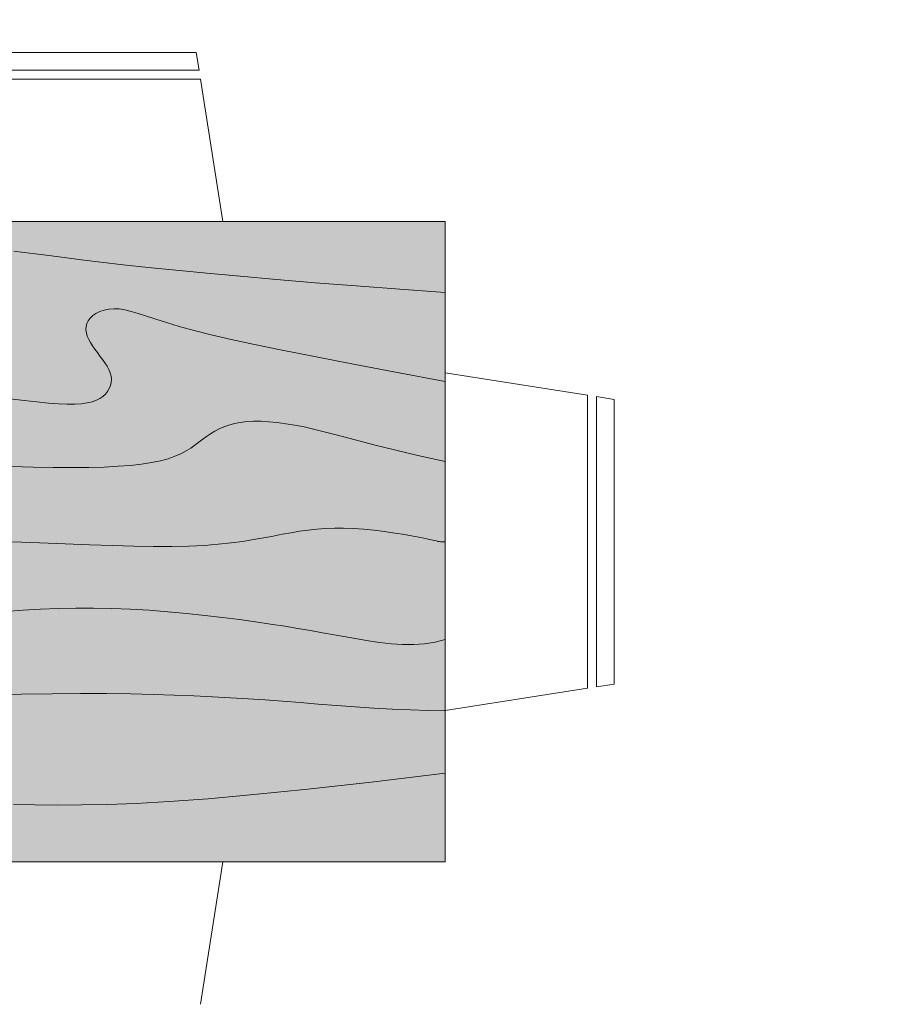
# Model space of a CAD drawing. Units: inches. Extents: x 2419 to 2878, y 1068 to 1713.
# Tile 6 of 20: x 2541 to 2574, y 1312 to 1349. Entities that reach past the tile are written whole.
import ezdxf

# ---------------------------------------------------------------- set-up
doc = ezdxf.new("R2010")
doc.units = ezdxf.units.IN
for name, color, linetype, lineweight in [('A-ANNO-DIMS', 2, 'Continuous', 18), ('A-FLOR-PRKG-PATT', 1, 'Continuous', 13), ('A-FURN', 8, 'Continuous', 18), ('A-FURN-PATT', 254, 'Continuous', 13)]:
    doc.layers.add(name, color=color, linetype=linetype, lineweight=lineweight)
doc.layers.add('A-WALL-PATT', color=18, linetype='Continuous', lineweight=13, true_color=0x000000)
doc.styles.get("Standard").update_dxf_attribs({"font": 'arial.ttf'})
doc.dimstyles.new('ISO-25', dxfattribs={"dimtxt": 12.5, "dimasz": 2.5, "dimexe": 1.25, "dimexo": 0.625, "dimtad": 1, "dimdec": 0, "dimlunit": 4, "dimtxsty": 'Standard', "dimblk": 'ARCHTICK', "dimcen": 2.5, "dimse1": 1, "dimse2": 1, "dimclrd": 4, "dimadec": 0, "dimazin": 0, "dimtfac": 1, "dimtdec": 0, "dimtmove": 0, "dimatfit": 3, "dimfxl": 1, "dimarcsym": 0})

# ---------------------------------------------------------------- blocks, each defined once
blk = doc.blocks.new('Dining Set - 36 x 72 in.')
for p, q in [((6, 27.5), (22, 27.5)), ((22.1563, 26.49966), (22, 27.5)), ((22.1584, 26.5), (5.8466, 26.5)), ((5.7696, 26), (22.2392, 26)), ((23.4848, 17.99762), (22.2345, 25.99926)), ((36, 18), (-36, 18)), ((36, -18), (36, 18)), ((44.0006, 8.23428), (35.9976, 9.48474)), ((44, 8.23041), (44, -8.23915)), ((44.5, -8.15843), (44.5, 8.15338)), ((45.5, 8), (44.5005, 8.15617)), ((45.5, 8), (45.5, -8)), ((35.9976, -9.48476), (43.9993, -8.2345)), ((44.4997, -8.15631), (45.5, -8)), ((-36, -18), (36, -18)), ((23.4848, -17.99762), (22.2345, -25.99928))]:
    blk.add_line(p, q)
for points in [[(11.75, 16.33333), (12.3184, 16.26318), (12.9694, 16.17838), (13.7151, 16.07991), (14.5677, 15.96875), (15.5395, 15.84586), (16.6426, 15.71224), (17.8893, 15.56884), (19.2917, 15.41666), (20.859, 15.25667), (22.5879, 15.08984), (24.4721, 14.91715), (26.5052, 14.73958), (28.6809, 14.5581), (30.9929, 14.3737), (33.4347, 14.18733), (36, 14)], [(11.5312, 8.03125), (12.3267, 7.93603), (13.043, 7.85547), (13.6831, 7.79248), (14.25, 7.75), (14.7471, 7.7303), (15.1797, 7.73307), (15.5537, 7.75732), (15.875, 7.80208), (16.1494, 7.86637), (16.3828, 7.94922), (16.5811, 8.04964), (16.75, 8.16666), (16.8944, 8.29915), (17.0143, 8.44531), (17.1089, 8.60319), (17.1771, 8.77083), (17.218, 8.94629), (17.2305, 9.1276), (17.2137, 9.31282), (17.1667, 9.5), (17.0895, 9.6875), (16.987, 9.875), (16.8649, 10.0625), (16.7292, 10.25), (16.5856, 10.4375), (16.4401, 10.625), (16.2985, 10.8125), (16.1667, 11), (16.05, 11.18733), (15.9518, 11.3737), (15.8752, 11.5581), (15.8229, 11.73958), (15.798, 11.91715), (15.8034, 12.08984), (15.842, 12.25667), (15.9167, 12.41666), (16.0295, 12.56836), (16.1784, 12.70833), (16.3605, 12.83268), (16.5729, 12.9375), (16.8127, 13.01888), (17.0768, 13.07291), (17.3625, 13.0957), (17.6667, 13.08333), (17.9894, 13.03312), (18.3418, 12.94726), (18.7382, 12.82918), (19.1927, 12.68229), (19.7195, 12.51001), (20.3327, 12.31575), (21.0465, 12.10294), (21.875, 11.875), (22.8357, 11.63354), (23.959, 11.37304), (25.2786, 11.08618), (26.8282, 10.76562), (28.6414, 10.40405), (30.752, 9.99414), (33.1936, 9.52856), (36, 9)], [(11.6309, 4.22819), (12.8281, 4.19531), (13.9551, 4.17415), (15, 4.16666), (15.954, 4.17448), (16.819, 4.19791), (17.6001, 4.23698), (18.3021, 4.29166), (18.9299, 4.36198), (19.4883, 4.44791), (19.9823, 4.54948), (20.4167, 4.66666), (20.7969, 4.79899), (21.1302, 4.94401), (21.4245, 5.09879), (21.6875, 5.26041), (21.9271, 5.42594), (22.1511, 5.59245), (22.3672, 5.757), (22.5834, 5.91666), (22.8065, 6.06868), (23.0404, 6.21093), (23.2879, 6.34147), (23.5521, 6.45833), (23.8358, 6.55957), (24.142, 6.64323), (24.4735, 6.70735), (24.8334, 6.75), (25.2235, 6.76969), (25.642, 6.76692), (26.0858, 6.74267), (26.5521, 6.69791), (27.0379, 6.63362), (27.5404, 6.55078), (28.0565, 6.45036), (28.5834, 6.33333), (29.1242, 6.19987), (29.7071, 6.04687), (30.3661, 5.87044), (31.1354, 5.66666), (32.0493, 5.43164), (33.142, 5.16146), (34.4475, 4.85221), (36, 4.5)], [(11.6667, 0), (13.1899, -0.06201), (14.6341, -0.1211), (15.9982, -0.17432), (17.2813, -0.21875), (18.4823, -0.25147), (19.6003, -0.26953), (20.6343, -0.27002), (21.5834, -0.25), (22.4481, -0.20768), (23.2357, -0.14584), (23.9549, -0.06836), (24.6146, 0.02083), (25.2235, 0.11784), (25.7904, 0.21875), (26.3241, 0.31966), (26.8334, 0.41666), (27.3265, 0.50618), (27.8099, 0.58593), (28.2894, 0.65397), (28.7709, 0.70833), (29.2601, 0.74707), (29.763, 0.76823), (30.2855, 0.76985), (30.8334, 0.75), (31.4088, 0.70784), (31.9994, 0.64713), (32.589, 0.57275), (33.1615, 0.48958), (33.7008, 0.4025), (34.1908, 0.3164), (34.6153, 0.23616), (34.9584, 0.16666), (35.2099, 0.11165), (35.3848, 0.07031), (35.504, 0.04069), (35.5886, 0.02083), (35.6594, 0.00879), (35.7377, 0.0026), (35.8442, 0.00032), (36, 0)], [(11.2734, -3.91407), (12.2647, -3.84603), (13.25, -3.79167), (14.2354, -3.75293), (15.2266, -3.73177), (16.2295, -3.73015), (17.25, -3.75), (18.2912, -3.79248), (19.3451, -3.85547), (20.4009, -3.93604), (21.4479, -4.03125), (22.4754, -4.13819), (23.4727, -4.25391), (24.4289, -4.37549), (25.3334, -4.5), (26.1785, -4.62492), (26.9694, -4.74935), (27.7145, -4.87281), (28.4219, -4.99479), (29.1, -5.11483), (29.7572, -5.23242), (30.4016, -5.34709), (31.0417, -5.45834), (31.6837, -5.56437), (32.3262, -5.65821), (32.9658, -5.73153), (33.599, -5.77604), (34.2224, -5.78345), (34.8327, -5.74545), (35.4264, -5.65373), (36, -5.5)], [(10.3021, -8.60677), (12.1712, -8.56543), (13.8958, -8.54167), (15.4876, -8.53353), (16.9583, -8.53907), (18.3197, -8.55632), (19.5834, -8.58334), (20.7616, -8.61841), (21.8685, -8.66081), (22.9188, -8.71004), (23.9271, -8.76563), (24.9081, -8.82707), (25.8763, -8.89388), (26.8465, -8.96558), (27.8334, -9.04167), (28.8474, -9.12118), (29.8828, -9.20117), (30.93, -9.27824), (31.9792, -9.34896), (33.0205, -9.40991), (34.0443, -9.45768), (35.0407, -9.48885), (36, -9.5)], [(11.7192, -14.76164), (12.929, -14.78711), (14.1965, -14.79794), (15.5417, -14.79167), (16.9933, -14.76424), (18.6152, -14.70508), (20.4804, -14.60197), (22.6615, -14.44271), (25.2312, -14.21509), (28.2624, -13.9069), (31.8277, -13.50594), (36, -13)]]:
    blk.add_lwpolyline(points)
blk = doc.blocks.new('_ArchTick')
at = {"color": 0, "linetype": 'ByBlock', "const_width": 0.15}
blk.add_lwpolyline([(-0.5, -0.5), (0.5, 0.5)], dxfattribs=at)
blk = doc.blocks.new('*D26')
at = {"layer": 'A-ANNO-DIMS', "color": 4, "lineweight": -2, "transparency": 16777216}
for p, q in [((2502.769, 1356.79), (2563.458, 1356.79)), ((2563.458, 1356.79), (2733.724, 1356.79))]:
    blk.add_line(p, q, dxfattribs=at)
at = {"layer": 'Defpoints', "color": 0, "transparency": 16777216}
for p in [(2563.458, 1356.79), (2502.769, 1347.687), (2563.458, 1347.687)]:
    blk.add_point(p, dxfattribs=at)
at = {"layer": 'A-ANNO-DIMS', "color": 4, "lineweight": -2, "transparency": 16777216, "xscale": 2.5, "yscale": 2.5, "zscale": 2.5, "rotation": 180}
blk.add_blockref('_ArchTick', (2502.769, 1356.79), dxfattribs=at)
at = {"layer": 'A-ANNO-DIMS', "color": 4, "lineweight": -2, "transparency": 16777216, "xscale": 2.5, "yscale": 2.5, "zscale": 2.5}
blk.add_blockref('_ArchTick', (2563.458, 1356.79), dxfattribs=at)
at = {"layer": 'A-ANNO-DIMS', "color": 0, "transparency": 16777216, "insert": (2649.841, 1363.878), "char_height": 12.5, "attachment_point": 5}
blk.add_mtext('DINING SET 5\'-0 1/2"', dxfattribs=at)
blk = doc.blocks.new('*D43')
at = {"layer": 'A-ANNO-DIMS', "color": 4, "lineweight": -2, "transparency": 16777216}
blk.add_line((2480.514, 1079.925), (2557.299, 1079.925), dxfattribs=at)
at = {"layer": 'Defpoints', "color": 0, "transparency": 16777216}
for p in [(2480.514, 1408.813), (2557.299, 1408.813), (2557.299, 1079.925)]:
    blk.add_point(p, dxfattribs=at)
at = {"layer": 'A-ANNO-DIMS', "color": 4, "lineweight": -2, "transparency": 16777216, "xscale": 2.5, "yscale": 2.5, "zscale": 2.5, "rotation": 180}
blk.add_blockref('_ArchTick', (2480.514, 1079.925), dxfattribs=at)
at = {"layer": 'A-ANNO-DIMS', "color": 4, "lineweight": -2, "transparency": 16777216, "xscale": 2.5, "yscale": 2.5, "zscale": 2.5}
blk.add_blockref('_ArchTick', (2557.299, 1079.925), dxfattribs=at)
at = {"layer": 'A-ANNO-DIMS', "color": 0, "transparency": 16777216, "insert": (2518.907, 1086.932), "char_height": 12.5, "attachment_point": 5}
blk.add_mtext('6\'-5"', dxfattribs=at)
blk = doc.blocks.new('*D44')
at = {"layer": 'A-ANNO-DIMS', "color": 4, "lineweight": -2, "transparency": 16777216}
for p, q in [((2557.299, 1079.925), (2585.818, 1079.925)), ((2585.818, 1079.925), (2652.136, 1079.925))]:
    blk.add_line(p, q, dxfattribs=at)
at = {"layer": 'Defpoints', "color": 0, "transparency": 16777216}
for p in [(2557.299, 1408.813), (2585.818, 1408.813), (2585.818, 1079.925)]:
    blk.add_point(p, dxfattribs=at)
at = {"layer": 'A-ANNO-DIMS', "color": 4, "lineweight": -2, "transparency": 16777216, "xscale": 2.5, "yscale": 2.5, "zscale": 2.5, "rotation": 180}
blk.add_blockref('_ArchTick', (2557.299, 1079.925), dxfattribs=at)
at = {"layer": 'A-ANNO-DIMS', "color": 4, "lineweight": -2, "transparency": 16777216, "xscale": 2.5, "yscale": 2.5, "zscale": 2.5}
blk.add_blockref('_ArchTick', (2585.818, 1079.925), dxfattribs=at)
at = {"layer": 'A-ANNO-DIMS', "color": 0, "transparency": 16777216, "insert": (2620.227, 1087.013), "char_height": 12.5, "attachment_point": 5}
blk.add_mtext('2\'-4 1/2"', dxfattribs=at)
blk = doc.blocks.new('*D47')
at = {"layer": 'A-ANNO-DIMS', "color": 4, "lineweight": -2, "transparency": 16777216}
for p, q in [((2444.314, 1376.561), (2444.314, 1357.976)), ((2444.314, 1357.976), (2444.314, 1293.048))]:
    blk.add_line(p, q, dxfattribs=at)
at = {"layer": 'Defpoints', "color": 0, "transparency": 16777216}
for p in [(2632.514, 1376.561), (2444.314, 1357.976), (2632.514, 1357.976)]:
    blk.add_point(p, dxfattribs=at)
at = {"layer": 'A-ANNO-DIMS', "color": 4, "lineweight": -2, "transparency": 16777216, "xscale": 2.5, "yscale": 2.5, "zscale": 2.5}
for p, rotation in [((2444.314, 1376.561), 90), ((2444.314, 1357.976), 270)]:
    blk.add_blockref('_ArchTick', p, dxfattribs=dict(at, rotation=rotation))
at = {"layer": 'A-ANNO-DIMS', "color": 0, "transparency": 16777216, "insert": (2437.226, 1324.262), "char_height": 12.5, "attachment_point": 5, "rotation": 90}
blk.add_mtext('1\'-6 1/2"', dxfattribs=at)
blk = doc.blocks.new('*D56')
at = {"layer": 'A-ANNO-DIMS', "color": 4, "lineweight": -2, "transparency": 16777216}
for p, q in [((2480.514, 1079.925), (2503.967, 1079.925)), ((2503.967, 1079.925), (2578.607, 1079.925))]:
    blk.add_line(p, q, dxfattribs=at)
at = {"layer": 'Defpoints', "color": 0, "transparency": 16777216}
for p in [(2480.514, 1507.813), (2503.967, 1494.852), (2503.967, 1079.925)]:
    blk.add_point(p, dxfattribs=at)
at = {"layer": 'A-ANNO-DIMS', "color": 4, "lineweight": -2, "transparency": 16777216, "xscale": 2.5, "yscale": 2.5, "zscale": 2.5, "rotation": 180}
blk.add_blockref('_ArchTick', (2480.514, 1079.925), dxfattribs=at)
at = {"layer": 'A-ANNO-DIMS', "color": 4, "lineweight": -2, "transparency": 16777216, "xscale": 2.5, "yscale": 2.5, "zscale": 2.5}
blk.add_blockref('_ArchTick', (2503.967, 1079.925), dxfattribs=at)
at = {"layer": 'A-ANNO-DIMS', "color": 0, "transparency": 16777216, "insert": (2542.537, 1087.013), "char_height": 12.5, "attachment_point": 5}
blk.add_mtext('1\'-11 1/2"', dxfattribs=at)
blk = doc.blocks.new('*D59')
at = {"layer": 'A-ANNO-DIMS', "color": 4, "lineweight": -2, "transparency": 16777216}
blk.add_line((2480.514, 1079.925), (2589.514, 1079.925), dxfattribs=at)
at = {"layer": 'Defpoints', "color": 0, "transparency": 16777216}
for p in [(2480.514, 1414.813), (2589.514, 1414.813), (2589.514, 1079.925)]:
    blk.add_point(p, dxfattribs=at)
at = {"layer": 'A-ANNO-DIMS', "color": 4, "lineweight": -2, "transparency": 16777216, "xscale": 2.5, "yscale": 2.5, "zscale": 2.5, "rotation": 180}
blk.add_blockref('_ArchTick', (2480.514, 1079.925), dxfattribs=at)
at = {"layer": 'A-ANNO-DIMS', "color": 4, "lineweight": -2, "transparency": 16777216, "xscale": 2.5, "yscale": 2.5, "zscale": 2.5}
blk.add_blockref('_ArchTick', (2589.514, 1079.925), dxfattribs=at)
at = {"layer": 'A-ANNO-DIMS', "color": 0, "transparency": 16777216, "insert": (2535.014, 1086.932), "char_height": 12.5, "attachment_point": 5}
blk.add_mtext('9\'-1"', dxfattribs=at)

msp = doc.modelspace()

# ---------------------------------------------------------------- hatches: boundary and pattern name
at = {"layer": 'A-FLOR-PRKG-PATT'}
h = msp.add_hatch(color=256, dxfattribs=at)
h.dxf.hatch_style = 1
edge = h.paths.add_edge_path()
edge.add_ellipse((2561.374, 1279.453), major_axis=(3.988, 0), ratio=0.842304, start_angle=0.6466, end_angle=90)
edge.add_line((2561.374, 1282.813), (2511.571, 1282.813))
edge.add_ellipse((2511.571, 1279.453), major_axis=(3.988, 0), ratio=0.842304, start_angle=90, end_angle=179.3534)
edge.add_ellipse((10560.892, 1188.617), major_axis=(-8054.031, 0), ratio=0.84230387, start_angle=-0.6465541, end_angle=-0.6282372)
edge.add_ellipse((2509.23, 1276.906), major_axis=(1.687, 0), ratio=0.842304, start_angle=179.3718, end_angle=248.4648)
edge.add_ellipse((10560.329, 1188.617), major_axis=(8052.293, 0), ratio=0.84230387, start_angle=179.3534459, end_angle=179.3813568, ccw=False)
edge.add_ellipse((2511.008, 1279.453), major_axis=(2.25, 0), ratio=0.842304, start_angle=90, end_angle=179.3534, ccw=False)
edge.add_line((2511.008, 1281.348), (2561.936, 1281.348))
edge.add_ellipse((2561.936, 1279.453), major_axis=(-2.25, 0), ratio=0.842304, start_angle=180.6466, end_angle=270, ccw=False)
edge.add_ellipse((-5487.385, 1188.617), major_axis=(8052.293, 0), ratio=0.84230387, start_angle=0.5282715, end_angle=0.6465541, ccw=False)
edge.add_ellipse((2563.715, 1276.906), major_axis=(-1.687, 0), ratio=0.842304, start_angle=111.5352, end_angle=180.6282)
edge.add_ellipse((-5487.947, 1188.617), major_axis=(-8054.031, 0), ratio=0.84230387, start_angle=180.6282372, end_angle=180.6465541)
edge = h.paths.add_edge_path()
edge.add_ellipse((2564.908, 1261.91), major_axis=(-1.125, 0), ratio=0.842304, start_angle=180, end_angle=270)
edge.add_line((2564.908, 1262.857), (2564.426, 1262.857))
edge.add_ellipse((-5487.385, 1188.617), major_axis=(8052.293, 0), ratio=0.84230387, start_angle=0.3838668, end_angle=0.5282715, ccw=False)
edge.add_line((2564.654, 1242.564), (2564.908, 1242.564))
edge.add_ellipse((2564.908, 1243.512), major_axis=(-1.125, 0), ratio=0.842304, start_angle=90, end_angle=180)
edge.add_line((2566.033, 1243.512), (2566.033, 1261.91))
edge = h.paths.add_edge_path()
edge.add_ellipse((2564.908, 1174.989), major_axis=(1.125, 0), ratio=0.842304, start_angle=0, end_angle=90)
edge.add_line((2564.908, 1175.936), (2564.894, 1175.936))
edge.add_ellipse((-5487.385, 1188.617), major_axis=(8052.293, 0), ratio=0.84230387, start_angle=-0.1349866, end_angle=-0.0902291, ccw=False)
edge.add_ellipse((2163.343, 1170.913), major_axis=(401.537, 0), ratio=0.8423039, start_angle=-2.17995, end_angle=-0.13561, ccw=False)
edge.add_line((2564.47, 1155.643), (2564.908, 1155.643))
edge.add_ellipse((2564.908, 1156.591), major_axis=(-1.125, 0), ratio=0.842304, start_angle=90, end_angle=180)
edge.add_line((2566.033, 1156.591), (2566.033, 1174.989))
h.paths.add_polyline_path([(2574.476, 1207.448), (2633.94, 1207.448), (2633.94, 1217.366), (2574.476, 1217.366)], flags=9)
h.paths.add_polyline_path([(2574.454, 1217.828), (2610.472, 1217.828), (2610.472, 1227.879), (2574.454, 1227.879)], flags=9)
h.paths.add_polyline_path([(2672.426, 1304.02), (2718.617, 1304.02), (2718.617, 1313.939), (2672.426, 1313.939)], flags=9)
h.paths.add_polyline_path([(2672.404, 1314.4), (2750.128, 1314.4), (2750.128, 1324.451), (2672.404, 1324.451)], flags=9)
h.paths.add_polyline_path([(2500.432, 1374.444), (2544.803, 1374.444), (2544.803, 1384.362), (2500.432, 1384.362)], flags=9)
h.paths.add_polyline_path([(2500.41, 1384.824), (2566.075, 1384.824), (2566.075, 1394.875), (2500.41, 1394.875)], flags=9)
h.paths.add_polyline_path([(2738.933, 1376.749), (2778.273, 1376.749), (2778.273, 1386.667), (2738.933, 1386.667)], flags=9)
h.paths.add_polyline_path([(2659.12, 1357.8), (2703.492, 1357.8), (2703.492, 1367.718), (2659.12, 1367.718)], flags=9)
h.paths.add_polyline_path([(2659.098, 1368.18), (2694.114, 1368.18), (2694.114, 1378.23), (2659.098, 1378.23)], flags=9)
h.paths.add_polyline_path([(2730.123, 1466.067), (2769.463, 1466.067), (2769.463, 1475.986), (2730.123, 1475.986)], flags=9)
h.paths.add_polyline_path([(2730.101, 1476.447), (2765.117, 1476.447), (2765.117, 1486.498), (2730.101, 1486.498)], flags=9)
h.paths.add_polyline_path([(2730.382, 1518.647), (2761.48, 1518.647), (2761.48, 1528.566), (2730.382, 1528.566)], flags=9)
h.paths.add_polyline_path([(2730.361, 1529.028), (2780.958, 1529.028), (2780.958, 1539.072), (2730.361, 1539.072)], flags=9)
h.paths.add_polyline_path([(2629.32, 1455.189), (2688.784, 1455.189), (2688.784, 1465.107), (2629.32, 1465.107)], flags=9)
h.paths.add_polyline_path([(2629.298, 1465.569), (2681.902, 1465.569), (2681.902, 1475.62), (2629.298, 1475.62)], flags=9)
h.paths.add_polyline_path([(2513.229, 1456.484), (2562.631, 1456.484), (2562.631, 1466.402), (2513.229, 1466.402)], flags=9)
h.paths.add_polyline_path([(2513.208, 1466.865), (2556.26, 1466.865), (2556.26, 1476.909), (2513.208, 1476.909)], flags=9)
h.paths.add_polyline_path([(2488.87, 1521.538), (2519.968, 1521.538), (2519.968, 1531.456), (2488.87, 1531.456)], flags=9)
h.paths.add_polyline_path([(2536.549, 1543.507), (2580.923, 1543.507), (2580.923, 1553.432), (2536.549, 1553.432)], flags=9)
h.paths.add_polyline_path([(2536.557, 1553.921), (2573.525, 1553.921), (2573.525, 1563.8), (2536.557, 1563.8)], flags=9)
at = {"layer": 'A-FURN-PATT'}
h = msp.add_hatch(color=256, dxfattribs=at)
h.dxf.hatch_style = 1
h.paths.add_polyline_path([(2541.329, 1340.193), (2541.763, 1340.136), (2542.26, 1340.071), (2542.829, 1339.996), (2543.477, 1339.914), (2544.213, 1339.825), (2545.044, 1339.73), (2545.979, 1339.628), (2547.025, 1339.521), (2548.178, 1339.41), (2549.434, 1339.295), (2550.79, 1339.177), (2552.241, 1339.056), (2553.783, 1338.933), (2555.412, 1338.808), (2557.123, 1338.683), (2557.123, 1341.351), (2509.104, 1341.351), (2509.104, 1339.35), (2512.321, 1339.335), (2515.235, 1339.293), (2517.872, 1339.227), (2520.258, 1339.142), (2522.419, 1339.041), (2524.38, 1338.928), (2526.167, 1338.808), (2527.806, 1338.683), (2529.318, 1338.559), (2530.71, 1338.437), (2531.983, 1338.32), (2533.138, 1338.211), (2534.177, 1338.112), (2535.102, 1338.027), (2535.914, 1337.957), (2536.615, 1337.905), (2537.208, 1337.874), (2537.702, 1337.862), (2538.108, 1337.868), (2538.435, 1337.891), (2538.695, 1337.93), (2538.897, 1337.983), (2539.052, 1338.05), (2539.171, 1338.128), (2539.263, 1338.216), (2539.33, 1338.313), (2539.376, 1338.416), (2539.401, 1338.524), (2539.407, 1338.634), (2539.398, 1338.745), (2539.374, 1338.855), (2539.338, 1338.961), (2539.292, 1339.063), (2539.238, 1339.16), (2539.211, 1339.204), (2538.872, 1339.739), (2539.045, 1340.125), (2539.381, 1340.287), (2539.76, 1340.325), (2540.185, 1340.315), (2540.752, 1340.264)])
h.paths.add_polyline_path([(2557.123, 1329.334), (2556.881, 1329.353), (2556.861, 1329.358), (2556.848, 1329.36), (2556.516, 1329.438), (2556.428, 1329.458), (2556.199, 1329.504), (2555.916, 1329.558), (2555.589, 1329.615), (2555.23, 1329.673), (2554.848, 1329.728), (2554.455, 1329.778), (2554.061, 1329.819), (2553.677, 1329.847), (2553.311, 1329.86), (2552.963, 1329.859), (2552.628, 1329.845), (2552.301, 1329.819), (2551.98, 1329.783), (2551.66, 1329.737), (2551.338, 1329.684), (2551.009, 1329.624), (2550.353, 1329.499), (2549.707, 1329.384), (2549.089, 1329.301), (2548.61, 1329.249), (2548.085, 1329.208), (2547.508, 1329.18), (2546.875, 1329.166), (2546.185, 1329.167), (2545.44, 1329.179), (2544.639, 1329.201), (2543.783, 1329.23), (2542.873, 1329.266), (2541.91, 1329.305), (2540.894, 1329.346), (2539.824, 1329.388), (2538.691, 1329.428), (2537.484, 1329.464), (2536.191, 1329.496), (2534.802, 1329.521), (2533.305, 1329.538), (2531.69, 1329.545), (2529.946, 1329.541), (2528.058, 1329.523), (2526.009, 1329.488), (2523.776, 1329.432), (2521.338, 1329.35), (2518.673, 1329.238), (2515.761, 1329.092), (2512.578, 1328.907), (2509.104, 1328.68), (2509.104, 1325.012), (2514.984, 1325.136), (2519.719, 1325.261), (2523.464, 1325.384), (2526.371, 1325.505), (2528.595, 1325.623), (2530.288, 1325.738), (2531.604, 1325.85), (2532.697, 1325.956), (2533.694, 1326.058), (2534.628, 1326.154), (2535.506, 1326.245), (2536.333, 1326.331), (2537.118, 1326.412), (2537.867, 1326.488), (2538.586, 1326.558), (2539.282, 1326.623), (2539.963, 1326.683), (2540.632, 1326.736), (2541.293, 1326.782), (2541.95, 1326.818), (2542.607, 1326.844), (2543.268, 1326.858), (2543.937, 1326.859), (2544.618, 1326.846), (2545.312, 1326.817), (2546.015, 1326.775), (2546.719, 1326.721), (2547.418, 1326.658), (2548.103, 1326.587), (2548.768, 1326.509), (2549.406, 1326.428), (2550.009, 1326.345), (2550.572, 1326.262), (2551.1, 1326.179), (2551.597, 1326.097), (2552.069, 1326.015), (2552.521, 1325.935), (2552.959, 1325.857), (2553.389, 1325.78), (2553.816, 1325.706), (2554.244, 1325.636), (2554.672, 1325.573), (2555.099, 1325.524), (2555.521, 1325.494), (2555.937, 1325.489), (2556.344, 1325.515), (2556.74, 1325.576), (2557.123, 1325.678)])
h.paths.add_polyline_path([(2557.123, 1335.349), (2555.251, 1335.701), (2553.623, 1336.012), (2552.215, 1336.285), (2551.006, 1336.526), (2549.972, 1336.74), (2549.092, 1336.931), (2548.343, 1337.105), (2547.702, 1337.266), (2547.15, 1337.418), (2546.674, 1337.56), (2546.265, 1337.69), (2545.913, 1337.805), (2545.61, 1337.903), (2545.346, 1337.981), (2545.111, 1338.039), (2544.896, 1338.072), (2544.693, 1338.08), (2544.502, 1338.065), (2544.326, 1338.029), (2544.166, 1337.975), (2544.025, 1337.905), (2543.903, 1337.822), (2543.804, 1337.729), (2543.729, 1337.627), (2543.679, 1337.521), (2543.653, 1337.409), (2543.649, 1337.294), (2543.666, 1337.176), (2543.701, 1337.055), (2543.752, 1336.932), (2543.818, 1336.808), (2543.895, 1336.683), (2543.983, 1336.558), (2544.078, 1336.433), (2544.175, 1336.307), (2544.271, 1336.182), (2544.361, 1336.057), (2544.442, 1335.932), (2544.511, 1335.807), (2544.562, 1335.682), (2544.594, 1335.557), (2544.605, 1335.434), (2544.597, 1335.313), (2544.569, 1335.196), (2544.524, 1335.084), (2544.461, 1334.979), (2544.381, 1334.881), (2544.284, 1334.793), (2544.172, 1334.715), (2544.039, 1334.648), (2543.884, 1334.593), (2543.701, 1334.55), (2543.487, 1334.52), (2543.237, 1334.504), (2542.949, 1334.502), (2542.617, 1334.515), (2542.239, 1334.543), (2541.812, 1334.585), (2541.334, 1334.639), (2540.804, 1334.703), (2540.219, 1334.774), (2539.577, 1334.851), (2538.876, 1334.932), (2538.115, 1335.015), (2537.292, 1335.099), (2536.409, 1335.183), (2535.465, 1335.268), (2534.465, 1335.356), (2533.408, 1335.446), (2532.297, 1335.539), (2531.133, 1335.636), (2529.918, 1335.738), (2528.635, 1335.843), (2527.193, 1335.945), (2525.484, 1336.036), (2523.398, 1336.106), (2520.826, 1336.148), (2517.659, 1336.152), (2513.788, 1336.111), (2509.104, 1336.016), (2509.104, 1333.015), (2512.629, 1332.904), (2515.728, 1332.821), (2518.445, 1332.76), (2520.824, 1332.716), (2522.909, 1332.685), (2524.743, 1332.663), (2526.37, 1332.645), (2527.834, 1332.626), (2529.173, 1332.602), (2530.407, 1332.574), (2531.551, 1332.542), (2532.62, 1332.507), (2533.63, 1332.47), (2534.594, 1332.43), (2535.529, 1332.389), (2536.448, 1332.348), (2537.364, 1332.306), (2538.272, 1332.266), (2539.164, 1332.228), (2540.033, 1332.195), (2540.87, 1332.166), (2541.669, 1332.144), (2542.42, 1332.13), (2543.117, 1332.125), (2543.754, 1332.131), (2544.33, 1332.146), (2544.851, 1332.172), (2545.32, 1332.209), (2545.738, 1332.256), (2546.111, 1332.313), (2546.44, 1332.381), (2546.73, 1332.459), (2546.983, 1332.547), (2547.206, 1332.644), (2547.402, 1332.747), (2547.577, 1332.855), (2547.737, 1332.965), (2547.886, 1333.076), (2548.031, 1333.186), (2548.175, 1333.292), (2548.324, 1333.394), (2548.48, 1333.489), (2548.645, 1333.576), (2548.821, 1333.654), (2549.01, 1333.721), (2549.214, 1333.777), (2549.435, 1333.82), (2549.675, 1333.848), (2549.936, 1333.861), (2550.215, 1333.859), (2550.511, 1333.843), (2550.822, 1333.813), (2551.146, 1333.771), (2551.481, 1333.715), (2551.825, 1333.648), (2552.176, 1333.57), (2552.537, 1333.481), (2552.926, 1333.379), (2553.365, 1333.262), (2553.878, 1333.126), (2554.488, 1332.969), (2555.217, 1332.789), (2556.087, 1332.583), (2557.123, 1332.348)])
h.paths.add_polyline_path([(2543.679, 1337.521), (2543.729, 1337.627), (2543.804, 1337.729), (2543.903, 1337.822), (2544.025, 1337.905), (2544.166, 1337.975), (2544.326, 1338.029), (2544.502, 1338.065), (2544.693, 1338.08), (2544.896, 1338.072), (2545.111, 1338.039), (2545.346, 1337.981), (2545.61, 1337.903), (2545.913, 1337.805), (2546.265, 1337.69), (2546.674, 1337.56), (2547.15, 1337.418), (2547.702, 1337.266), (2548.343, 1337.105), (2549.092, 1336.931), (2549.972, 1336.74), (2551.006, 1336.526), (2552.215, 1336.285), (2553.623, 1336.012), (2555.251, 1335.701), (2557.123, 1335.349), (2557.123, 1338.683), (2555.412, 1338.808), (2553.783, 1338.933), (2552.241, 1339.056), (2550.79, 1339.177), (2549.434, 1339.295), (2548.178, 1339.41), (2547.025, 1339.521), (2545.979, 1339.628), (2545.044, 1339.73), (2544.213, 1339.825), (2543.477, 1339.914), (2542.829, 1339.996), (2542.26, 1340.071), (2541.763, 1340.136), (2541.329, 1340.193), (2540.95, 1340.24), (2540.618, 1340.276), (2540.33, 1340.302), (2540.08, 1340.318), (2539.866, 1340.323), (2539.683, 1340.318), (2539.527, 1340.302), (2539.395, 1340.276), (2539.282, 1340.24), (2539.186, 1340.193), (2539.105, 1340.137), (2539.04, 1340.073), (2538.991, 1340.003), (2538.957, 1339.928), (2538.939, 1339.849), (2538.936, 1339.767), (2538.949, 1339.684), (2538.977, 1339.6), (2539.018, 1339.516), (2539.067, 1339.431), (2539.123, 1339.343), (2539.222, 1339.189), (2539.323, 1339.007), (2539.374, 1338.855), (2539.398, 1338.745), (2539.407, 1338.634), (2539.401, 1338.524), (2539.376, 1338.416), (2539.33, 1338.313), (2539.263, 1338.216), (2539.171, 1338.128), (2539.052, 1338.05), (2538.897, 1337.983), (2538.695, 1337.93), (2538.435, 1337.891), (2538.108, 1337.868), (2537.702, 1337.862), (2537.208, 1337.874), (2536.615, 1337.905), (2535.914, 1337.957), (2535.102, 1338.027), (2534.177, 1338.112), (2533.138, 1338.211), (2531.983, 1338.32), (2530.71, 1338.437), (2529.318, 1338.559), (2527.806, 1338.683), (2526.167, 1338.808), (2524.38, 1338.928), (2522.419, 1339.041), (2520.258, 1339.142), (2517.872, 1339.227), (2515.235, 1339.293), (2512.321, 1339.335), (2509.104, 1339.35), (2509.104, 1336.016), (2513.788, 1336.111), (2517.659, 1336.152), (2520.826, 1336.148), (2523.398, 1336.106), (2525.484, 1336.036), (2527.193, 1335.945), (2528.635, 1335.843), (2529.918, 1335.738), (2531.133, 1335.636), (2532.297, 1335.539), (2533.408, 1335.446), (2534.465, 1335.356), (2535.465, 1335.268), (2536.409, 1335.183), (2537.292, 1335.099), (2538.115, 1335.015), (2538.876, 1334.932), (2539.577, 1334.851), (2540.219, 1334.774), (2540.804, 1334.703), (2541.334, 1334.639), (2541.812, 1334.585), (2542.239, 1334.543), (2542.617, 1334.515), (2542.949, 1334.502), (2543.237, 1334.504), (2543.487, 1334.52), (2543.701, 1334.55), (2543.884, 1334.593), (2544.039, 1334.648), (2544.172, 1334.715), (2544.284, 1334.793), (2544.381, 1334.881), (2544.461, 1334.979), (2544.524, 1335.084), (2544.569, 1335.196), (2544.597, 1335.313), (2544.605, 1335.434), (2544.594, 1335.557), (2544.562, 1335.682), (2544.511, 1335.807), (2544.442, 1335.932), (2544.361, 1336.057), (2544.271, 1336.182), (2544.175, 1336.307), (2544.078, 1336.433), (2543.983, 1336.558), (2543.895, 1336.683), (2543.818, 1336.808), (2543.752, 1336.932), (2543.701, 1337.055), (2543.666, 1337.176), (2543.649, 1337.294), (2543.653, 1337.409)])
h.paths.add_polyline_path([(2557.123, 1332.348), (2556.087, 1332.583), (2555.217, 1332.789), (2554.488, 1332.969), (2553.878, 1333.126), (2553.365, 1333.262), (2552.926, 1333.379), (2552.537, 1333.481), (2552.176, 1333.57), (2551.825, 1333.648), (2551.481, 1333.715), (2551.146, 1333.771), (2550.822, 1333.813), (2550.511, 1333.843), (2550.215, 1333.859), (2549.936, 1333.861), (2549.675, 1333.848), (2549.435, 1333.82), (2549.214, 1333.777), (2549.01, 1333.721), (2548.821, 1333.654), (2548.645, 1333.576), (2548.48, 1333.489), (2548.324, 1333.394), (2548.175, 1333.292), (2548.031, 1333.186), (2547.886, 1333.076), (2547.737, 1332.965), (2547.577, 1332.855), (2547.402, 1332.747), (2547.206, 1332.644), (2546.983, 1332.547), (2546.73, 1332.459), (2546.44, 1332.381), (2546.111, 1332.313), (2545.738, 1332.256), (2545.32, 1332.209), (2544.851, 1332.172), (2544.33, 1332.146), (2543.754, 1332.131), (2543.117, 1332.125), (2542.42, 1332.13), (2541.669, 1332.144), (2540.87, 1332.166), (2540.033, 1332.195), (2539.164, 1332.228), (2538.272, 1332.266), (2537.364, 1332.306), (2536.448, 1332.348), (2535.529, 1332.389), (2534.594, 1332.43), (2533.63, 1332.47), (2532.62, 1332.507), (2531.551, 1332.542), (2530.407, 1332.574), (2529.173, 1332.602), (2527.834, 1332.626), (2526.37, 1332.645), (2524.743, 1332.663), (2522.909, 1332.685), (2520.824, 1332.716), (2518.445, 1332.76), (2515.728, 1332.821), (2512.629, 1332.904), (2509.104, 1333.015), (2509.104, 1328.68), (2512.578, 1328.907), (2515.761, 1329.092), (2518.673, 1329.238), (2521.338, 1329.35), (2523.776, 1329.432), (2526.009, 1329.488), (2528.058, 1329.523), (2529.946, 1329.541), (2531.69, 1329.545), (2533.305, 1329.538), (2534.802, 1329.521), (2536.191, 1329.496), (2537.484, 1329.464), (2538.691, 1329.428), (2539.824, 1329.388), (2540.894, 1329.346), (2541.91, 1329.305), (2542.873, 1329.266), (2543.783, 1329.23), (2544.639, 1329.201), (2545.44, 1329.179), (2546.185, 1329.167), (2546.875, 1329.166), (2547.508, 1329.18), (2548.085, 1329.208), (2548.61, 1329.249), (2549.089, 1329.301), (2549.529, 1329.36), (2549.936, 1329.425), (2550.314, 1329.492), (2550.67, 1329.56), (2551.009, 1329.624), (2551.338, 1329.684), (2551.66, 1329.737), (2551.98, 1329.783), (2552.301, 1329.819), (2552.628, 1329.845), (2552.963, 1329.859), (2553.311, 1329.86), (2553.677, 1329.847), (2554.061, 1329.819), (2554.455, 1329.778), (2554.848, 1329.728), (2555.23, 1329.673), (2555.589, 1329.615), (2555.916, 1329.558), (2556.199, 1329.504), (2556.428, 1329.458), (2556.596, 1329.421), (2556.712, 1329.393), (2556.792, 1329.374), (2556.848, 1329.36), (2556.895, 1329.352), (2556.948, 1329.348), (2557.019, 1329.347), (2557.123, 1329.346)])
h.paths.add_polyline_path([(2557.123, 1323.011), (2556.483, 1323.018), (2555.818, 1323.039), (2555.136, 1323.071), (2554.441, 1323.111), (2553.741, 1323.159), (2553.043, 1323.21), (2552.352, 1323.263), (2551.676, 1323.316), (2551.018, 1323.367), (2550.371, 1323.415), (2549.725, 1323.46), (2549.071, 1323.501), (2548.398, 1323.538), (2547.698, 1323.57), (2546.96, 1323.599), (2546.174, 1323.622), (2545.331, 1323.64), (2544.423, 1323.652), (2543.442, 1323.655), (2542.381, 1323.65), (2541.231, 1323.634), (2539.984, 1323.606), (2538.633, 1323.566), (2537.171, 1323.511), (2535.566, 1323.441), (2533.7, 1323.357), (2531.431, 1323.262), (2528.619, 1323.157), (2525.121, 1323.044), (2520.797, 1322.925), (2515.505, 1322.802), (2509.104, 1322.677), (2509.104, 1319.676), (2513.047, 1319.786), (2516.418, 1319.868), (2519.287, 1319.925), (2521.724, 1319.961), (2523.797, 1319.978), (2525.575, 1319.981), (2527.13, 1319.972), (2528.528, 1319.954), (2529.831, 1319.931), (2531.052, 1319.903), (2532.199, 1319.871), (2533.277, 1319.836), (2534.29, 1319.798), (2535.246, 1319.759), (2536.148, 1319.718), (2537.004, 1319.676), (2537.819, 1319.635), (2538.606, 1319.595), (2539.377, 1319.558), (2540.147, 1319.527), (2540.929, 1319.502), (2541.736, 1319.485), (2542.581, 1319.477), (2543.479, 1319.482), (2544.447, 1319.5), (2545.528, 1319.539), (2546.772, 1319.608), (2548.227, 1319.714), (2549.941, 1319.866), (2551.962, 1320.072), (2554.34, 1320.339), (2557.123, 1320.677)], flags=17)
h.paths.add_polyline_path([(2557.123, 1325.678), (2556.74, 1325.576), (2556.344, 1325.515), (2555.937, 1325.489), (2555.521, 1325.494), (2555.099, 1325.524), (2554.672, 1325.573), (2554.244, 1325.636), (2553.816, 1325.706), (2553.389, 1325.78), (2552.959, 1325.857), (2552.521, 1325.935), (2552.069, 1326.015), (2551.597, 1326.097), (2551.1, 1326.179), (2550.572, 1326.262), (2550.009, 1326.345), (2549.406, 1326.428), (2548.768, 1326.509), (2548.103, 1326.587), (2547.418, 1326.658), (2546.719, 1326.721), (2546.015, 1326.775), (2545.312, 1326.817), (2544.618, 1326.846), (2543.937, 1326.859), (2543.268, 1326.858), (2542.607, 1326.844), (2541.95, 1326.818), (2541.293, 1326.782), (2540.632, 1326.736), (2539.963, 1326.683), (2539.282, 1326.623), (2538.586, 1326.558), (2537.867, 1326.488), (2537.118, 1326.412), (2536.333, 1326.331), (2535.506, 1326.245), (2534.628, 1326.154), (2533.694, 1326.058), (2532.697, 1325.956), (2531.604, 1325.85), (2530.288, 1325.738), (2528.595, 1325.623), (2526.371, 1325.505), (2523.464, 1325.384), (2519.719, 1325.261), (2514.984, 1325.136), (2509.104, 1325.012), (2509.104, 1319.676), (2513.047, 1319.786), (2516.418, 1319.868), (2519.287, 1319.925), (2521.724, 1319.961), (2523.797, 1319.978), (2525.575, 1319.981), (2527.13, 1319.972), (2528.528, 1319.954), (2529.831, 1319.931), (2531.052, 1319.903), (2532.199, 1319.871), (2533.277, 1319.836), (2534.29, 1319.798), (2535.246, 1319.759), (2536.148, 1319.718), (2537.004, 1319.676), (2537.819, 1319.635), (2538.606, 1319.595), (2539.377, 1319.558), (2540.147, 1319.527), (2540.929, 1319.502), (2541.736, 1319.485), (2542.581, 1319.477), (2543.479, 1319.482), (2544.447, 1319.5), (2545.528, 1319.539), (2546.772, 1319.608), (2548.227, 1319.714), (2549.941, 1319.866), (2551.962, 1320.072), (2554.34, 1320.339), (2557.123, 1320.677)])
h.paths.add_polyline_path([(2557.123, 1320.677), (2554.34, 1320.339), (2551.962, 1320.072), (2549.941, 1319.866), (2548.227, 1319.714), (2546.772, 1319.608), (2545.528, 1319.539), (2544.447, 1319.5), (2543.479, 1319.482), (2542.581, 1319.477), (2541.736, 1319.485), (2540.929, 1319.502), (2540.147, 1319.527), (2539.377, 1319.558), (2538.606, 1319.595), (2537.819, 1319.635), (2537.004, 1319.676), (2536.148, 1319.718), (2535.246, 1319.759), (2534.29, 1319.798), (2533.277, 1319.836), (2532.199, 1319.871), (2531.052, 1319.903), (2529.831, 1319.931), (2528.528, 1319.954), (2527.13, 1319.972), (2525.575, 1319.981), (2523.797, 1319.978), (2521.724, 1319.961), (2519.287, 1319.925), (2516.418, 1319.868), (2513.047, 1319.786), (2509.104, 1319.676), (2509.104, 1317.342), (2557.123, 1317.342)])
h = msp.add_hatch(color=256, dxfattribs=at)
h.dxf.hatch_style = 1
h.paths.add_polyline_path([(2557.123, 1323.011), (2556.483, 1323.018), (2555.818, 1323.039), (2555.136, 1323.071), (2554.441, 1323.111), (2553.741, 1323.159), (2553.043, 1323.21), (2552.352, 1323.263), (2551.676, 1323.316), (2551.018, 1323.367), (2550.371, 1323.415), (2549.725, 1323.46), (2549.071, 1323.501), (2548.398, 1323.538), (2547.698, 1323.57), (2546.96, 1323.599), (2546.174, 1323.622), (2545.331, 1323.64), (2544.423, 1323.652), (2543.442, 1323.655), (2542.381, 1323.65), (2541.231, 1323.634), (2539.984, 1323.606), (2538.633, 1323.566), (2537.171, 1323.511), (2535.566, 1323.441), (2533.7, 1323.357), (2531.431, 1323.262), (2528.619, 1323.157), (2525.121, 1323.044), (2520.797, 1322.925), (2515.505, 1322.802), (2509.104, 1322.677), (2509.104, 1319.676), (2513.047, 1319.786), (2516.418, 1319.868), (2519.287, 1319.925), (2521.724, 1319.961), (2523.797, 1319.978), (2525.575, 1319.981), (2527.13, 1319.972), (2528.528, 1319.954), (2529.831, 1319.931), (2531.052, 1319.903), (2532.199, 1319.871), (2533.277, 1319.836), (2534.29, 1319.798), (2535.246, 1319.759), (2536.148, 1319.718), (2537.004, 1319.676), (2537.819, 1319.635), (2538.606, 1319.595), (2539.377, 1319.558), (2540.147, 1319.527), (2540.929, 1319.502), (2541.736, 1319.485), (2542.581, 1319.477), (2543.479, 1319.482), (2544.447, 1319.5), (2545.528, 1319.539), (2546.772, 1319.608), (2548.227, 1319.714), (2549.941, 1319.866), (2551.962, 1320.072), (2554.34, 1320.339), (2557.123, 1320.677)])
at = {"layer": 'A-WALL-PATT'}
h = msp.add_hatch(color=256, dxfattribs=at)
h.dxf.hatch_style = 1
h.paths.add_polyline_path([(2780.514, 1577.813), (2471.514, 1577.813), (2471.514, 1121.813), (2780.514, 1121.813)])
h.paths.add_polyline_path([(2480.514, 1568.813), (2771.514, 1568.813), (2771.514, 1130.813), (2480.514, 1130.813)], flags=16)
h.paths.add_polyline_path([(2528.514, 1568.813), (2528.514, 1512.813), (2594.514, 1512.813), (2594.514, 1414.813), (2596.568, 1414.813), (2596.568, 1441.609), (2597.816, 1441.609), (2597.816, 1441.582, -0.384016), (2625.035, 1414.813), (2725.514, 1414.813), (2725.514, 1567.545), (2728.302, 1567.545), (2746.887, 1567.545), (2746.887, 1566.732), (2746.87, 1566.732, -0.367216), (2730.514, 1549.092), (2730.514, 1512.813), (2750.853, 1512.813), (2750.853, 1510.025, -0.401453), (2733.081, 1491.458), (2733.081, 1491.44), (2732.268, 1491.44), (2732.268, 1507.813), (2730.514, 1507.813), (2730.514, 1408.813), (2736.514, 1408.813), (2736.514, 1349.813), (2632.514, 1349.813), (2632.514, 1408.813), (2528.514, 1408.813), (2528.514, 1414.813), (2503.967, 1414.813), (2503.967, 1494.852), (2558.379, 1494.852), (2558.379, 1507.813), (2529.965, 1507.813, -0.414214), (2530.821, 1506.957), (2530.821, 1497.257, -0.414214), (2529.965, 1496.401), (2514.559, 1496.401, -0.414214), (2513.703, 1497.257), (2513.703, 1506.957, -0.414214), (2514.559, 1507.813), (2528.514, 1507.813), (2528.514, 1512.813), (2480.514, 1512.813)], flags=0)
h.paths.add_polyline_path([(2516.262, 1507.813), (2528.262, 1507.813), (2528.262, 1505.813), (2523.417, 1505.813), (2524.074, 1504.675), (2529.394, 1504.675, -0.414214), (2529.965, 1504.104), (2529.965, 1497.828, -0.414214), (2529.394, 1497.257), (2515.13, 1497.257, -0.414214), (2514.559, 1497.828), (2514.559, 1504.104, -0.414214), (2515.13, 1504.675), (2520.689, 1504.675), (2521.342, 1505.813), (2516.262, 1505.813)], flags=0)
h.paths.add_polyline_path([(2522.016, 1505.531), (2522.817, 1507.318, -0.65506), (2522.254, 1506.063), (2522.195, 1505.93), (2522.425, 1505.531)], flags=0)
h.paths.add_polyline_path([(2522.833, 1500.966, -1), (2521.691, 1500.966, -1)], flags=0)
h.paths.add_polyline_path([(2522.547, 1500.966, -1), (2521.977, 1500.966, -1)], flags=0)
h.paths.add_polyline_path([(2482.005, 1470.633), (2499.894, 1470.633), (2499.894, 1448.272), (2482.005, 1448.272), (2482.005, 1452.744), (2481.26, 1452.744), (2481.26, 1449.763), (2480.514, 1449.763), (2480.514, 1469.142), (2481.26, 1469.142), (2481.26, 1466.16), (2482.005, 1466.16)], flags=0)
h.paths.add_polyline_path([(2488.713, 1466.16, -1), (2484.241, 1466.16, -1)], flags=0)
h.paths.add_polyline_path([(2496.167, 1466.16, -1), (2490.204, 1466.16, -1)], flags=0)
h.paths.add_polyline_path([(2487.968, 1466.16, -1), (2484.987, 1466.16, -1)], flags=0)
h.paths.add_polyline_path([(2495.422, 1466.16, -1), (2490.949, 1466.16, -1)], flags=0)
h.paths.add_polyline_path([(2487.223, 1466.16, -1), (2485.732, 1466.16, -1)], flags=0)
h.paths.add_polyline_path([(2494.676, 1466.16, -1), (2491.695, 1466.16, -1)], flags=0)
h.paths.add_polyline_path([(2499.108, 1468.005, -1), (2497.977, 1468.005, -1)], flags=0)
h.paths.add_polyline_path([(2493.931, 1466.16, -1), (2492.44, 1466.16, -1)], flags=0)
h.paths.add_polyline_path([(2499.372, 1463.71, -1), (2498.166, 1463.71, -1)], flags=0)
h.paths.add_polyline_path([(2484.241, 1461.688), (2496.167, 1461.688), (2496.167, 1457.216), (2484.241, 1457.216)], flags=0)
h.paths.add_polyline_path([(2484.987, 1460.943), (2495.422, 1460.943), (2495.422, 1457.961), (2484.987, 1457.961)], flags=0)
h.paths.add_polyline_path([(2586.88, 1510.025), (2587.693, 1510.025), (2587.693, 1491.44), (2586.88, 1491.44)], flags=0)
h.paths.add_polyline_path([(2499.259, 1459.415, -1), (2498.203, 1459.415, -1)], flags=0)
h.paths.add_polyline_path([(2489.459, 1452.744, -1), (2483.496, 1452.744, -1)], flags=0)
h.paths.add_polyline_path([(2557.299, 1408.813), (2557.299, 1413.091, -0.401453), (2584.57, 1441.582), (2584.57, 1441.609), (2585.818, 1441.609), (2585.818, 1413.091), (2585.818, 1408.813)], flags=0)
h.paths.add_polyline_path([(2488.713, 1452.744, -1), (2484.241, 1452.744, -1)], flags=0)
h.paths.add_polyline_path([(2495.422, 1452.744, -1), (2490.949, 1452.744, -1)], flags=0)
h.paths.add_polyline_path([(2487.968, 1452.744, -1), (2484.987, 1452.744, -1)], flags=0)
h.paths.add_polyline_path([(2494.676, 1452.744, -1), (2491.695, 1452.744, -1)], flags=0)
h.paths.add_polyline_path([(2487.223, 1452.744, -1), (2485.732, 1452.744, -1)], flags=0)
h.paths.add_polyline_path([(2499.183, 1454.442, -1), (2497.902, 1454.442, -1)], flags=0)
h.paths.add_polyline_path([(2493.931, 1452.744, -1), (2492.44, 1452.744, -1)], flags=0)
h.paths.add_polyline_path([(2499.296, 1450.637, -1), (2497.789, 1450.637, -1)], flags=0)
h.paths.add_polyline_path([(2619.129, 1558.889, -1), (2605.129, 1558.889, -1)], flags=0)
h.paths.add_polyline_path([(2609.129, 1558.889), (2612.129, 1561.889), (2615.129, 1558.889), (2612.129, 1555.889)], flags=0)
h.paths.add_polyline_path([(2611.129, 1558.889, -1), (2613.129, 1558.889, -1)], flags=0)
h.paths.add_polyline_path([(2633.679, 1568.813), (2693.679, 1568.813), (2693.679, 1488.813), (2633.679, 1488.813)], flags=0)
h.paths.add_polyline_path([(2641.679, 1554.413), (2641.679, 1567.613), (2662.479, 1567.613), (2662.479, 1554.413), (2664.879, 1554.413), (2664.879, 1567.613), (2685.679, 1567.613), (2685.679, 1552.413), (2680.479, 1552.413), (2693.679, 1539.213), (2678.479, 1539.213), (2678.479, 1554.413)], flags=0)
h.paths.add_polyline_path([(2637.514, 1408.813), (2731.514, 1408.813), (2731.514, 1354.813), (2637.514, 1354.813), (2637.514, 1357.976), (2635.302, 1357.976), (2635.302, 1358.789), (2637.514, 1358.789)], flags=0)
h.paths.add_polyline_path([(2717.171, 1559.643, -1), (2703.171, 1559.643, -1)], flags=0)
h.paths.add_polyline_path([(2707.171, 1559.643), (2710.171, 1562.643), (2713.171, 1559.643), (2710.171, 1556.643)], flags=0)
h.paths.add_polyline_path([(2709.171, 1559.643, -1), (2711.171, 1559.643, -1)], flags=0)
h.paths.add_polyline_path([(2685.378, 1408.813), (2706.378, 1408.813), (2706.378, 1400.813), (2699.878, 1400.813), (2701.878, 1394.813, -0.501323), (2696.923, 1375.952, -0.132891), (2694.834, 1375.952, -0.501317), (2689.878, 1394.813), (2691.878, 1400.813), (2688.878, 1400.813), (2688.878, 1399.313), (2685.878, 1399.313), (2685.878, 1400.313), (2687.878, 1400.313), (2687.878, 1400.813), (2685.378, 1400.813)], flags=0)
h.paths.add_polyline_path([(2687.378, 1407.813), (2704.378, 1407.813, -0.5), (2705.378, 1406.813), (2705.378, 1402.813, -0.5), (2704.378, 1401.813), (2687.378, 1401.813, -0.5), (2686.378, 1402.813), (2686.378, 1406.813, -0.5)], flags=0)
h.paths.add_polyline_path([(2639.514, 1205.813), (2634.514, 1205.813), (2634.514, 1293.813), (2637.514, 1293.813), (2639.514, 1293.813)], flags=0)
h.paths.add_polyline_path([(2691.878, 1394.813), (2699.878, 1394.813, -0.48008), (2697.522, 1377.29, -0.215004), (2694.234, 1377.29, -0.48008)], flags=0)
h.paths.add_polyline_path([(2757.514, 1453.891), (2763.514, 1451.891), (2763.514, 1454.891), (2762.014, 1454.891), (2762.014, 1457.891), (2763.014, 1457.891), (2763.014, 1455.891), (2763.514, 1455.891), (2763.514, 1458.391), (2771.514, 1458.391), (2771.514, 1437.391), (2763.514, 1437.391), (2763.514, 1443.891), (2757.515, 1441.891, -0.501323), (2738.653, 1446.847, -0.132891), (2738.653, 1448.936, -0.501317)], flags=0)
h.paths.add_polyline_path([(2739.991, 1449.535, -0.48008), (2757.514, 1451.891), (2757.514, 1443.891, -0.48008), (2739.991, 1446.247, -0.215004)], flags=0)
h.paths.add_polyline_path([(2765.514, 1457.391), (2769.514, 1457.391, -0.5), (2770.514, 1456.391), (2770.514, 1439.391, -0.5), (2769.514, 1438.391), (2765.514, 1438.391, -0.5), (2764.514, 1439.391), (2764.514, 1456.391, -0.5)], flags=0)

# ---------------------------------------------------------------- block references
at = {"layer": 'A-FURN', "xscale": 0.6669202688727635, "yscale": 0.6669202688727635, "zscale": 0.6669202688727635}
msp.add_blockref('Dining Set - 36 x 72 in.', (2533.113, 1329.346), dxfattribs=at)

# ---------------------------------------------------------------- dimensions: what is measured, and where the dimension line sits
at = {"layer": 'A-ANNO-DIMS'}
for base, p1, p2, picture, middle in [((2503.967, 1079.925), (2480.514, 1507.813), (2503.967, 1494.852), '*D56', (2542.537, 1087.013)), ((2589.514, 1079.925), (2480.514, 1414.813), (2589.514, 1414.813), '*D59', (2535.014, 1086.932)), ((2557.299, 1079.925), (2480.514, 1408.813), (2557.299, 1408.813), '*D43', (2518.907, 1086.932)), ((2585.818, 1079.925), (2557.299, 1408.813), (2585.818, 1408.813), '*D44', (2620.227, 1087.013))]:
    dim = msp.add_linear_dim(base=base, p1=p1, p2=p2, dimstyle='ISO-25', override={"dimdec": 1, "dimlfac": 1, "dimrnd": 0, "dimzin": 1, "dimdsep": 46, "dimlunit": 4, "dimfrac": 2}, dxfattribs=at)
    dim.commit()
    dim.dimension.update_dxf_attribs({"geometry": picture, "text_midpoint": middle})
dim = msp.add_linear_dim(base=(2563.458, 1356.79), p1=(2502.769, 1347.687), p2=(2563.458, 1347.687), text='DINING SET <>', dimstyle='ISO-25', override={"dimdec": 1, "dimlfac": 1, "dimrnd": 0, "dimzin": 1, "dimdsep": 46, "dimlunit": 4, "dimfrac": 2}, dxfattribs=at)
dim.commit()
dim.dimension.update_dxf_attribs({"geometry": '*D26', "text_midpoint": (2649.841, 1363.878)})
dim = msp.add_linear_dim(base=(2444.314, 1357.976), p1=(2632.514, 1376.561), p2=(2632.514, 1357.976), angle=90, dimstyle='ISO-25', override={"dimdec": 1, "dimlfac": 1, "dimrnd": 0, "dimzin": 1, "dimdsep": 46, "dimlunit": 4, "dimfrac": 2}, dxfattribs=at)
dim.commit()
dim.dimension.update_dxf_attribs({"geometry": '*D47', "text_midpoint": (2437.226, 1324.262)})

doc.saveas('drawing.dxf')
